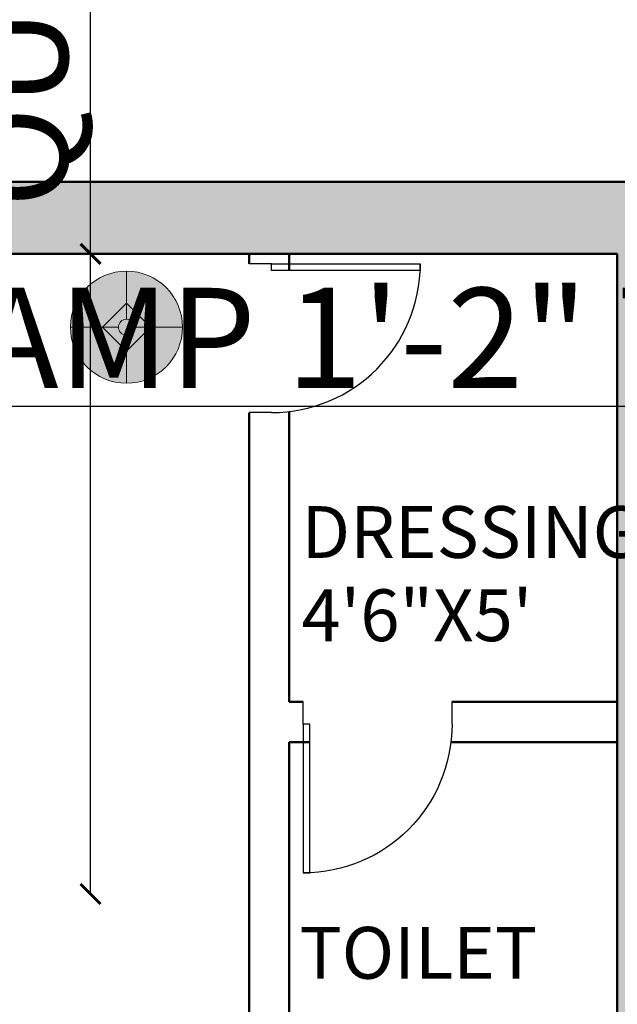
# Model space of a CAD drawing. Units: inches. Extents: x 2419 to 2878, y 1068 to 1713.
# Tile 18 of 20: x 2697 to 2772, y 1475 to 1598. Entities that reach past the tile are written whole.
import ezdxf

# ---------------------------------------------------------------- set-up
doc = ezdxf.new("R2010")
doc.units = ezdxf.units.IN
for name, color, linetype, lineweight in [('A-ANNO-DIMS', 2, 'Continuous', 18), ('A-AREA-IDEN', 7, 'Continuous', 18), ('A-DOOR', 4, 'Continuous', 25), ('A-FLOR-PRKG-PATT', 1, 'Continuous', 13), ('A-FURN', 8, 'Continuous', 18), ('A-FURN-PATT', 254, 'Continuous', 13), ('A-WALL', 7, 'Continuous', 50)]:
    doc.layers.add(name, color=color, linetype=linetype, lineweight=lineweight)
doc.layers.add('A-FLOR-FIXT-PATT', color=254, linetype='Continuous', lineweight=13, true_color=0xd7ebd2)
doc.layers.add('A-WALL-PATT', color=18, linetype='Continuous', lineweight=13, true_color=0x000000)
doc.styles.get("Standard").update_dxf_attribs({"font": 'arial.ttf'})
doc.dimstyles.new('ISO-25', dxfattribs={"dimtxt": 12.5, "dimasz": 2.5, "dimexe": 1.25, "dimexo": 0.625, "dimtad": 1, "dimdec": 0, "dimlunit": 4, "dimtxsty": 'Standard', "dimblk": 'ARCHTICK', "dimcen": 2.5, "dimse1": 1, "dimse2": 1, "dimclrd": 4, "dimadec": 0, "dimazin": 0, "dimtfac": 1, "dimtdec": 0, "dimtmove": 0, "dimatfit": 3, "dimfxl": 1, "dimarcsym": 0})

# ---------------------------------------------------------------- blocks, each defined once
blk = doc.blocks.new('*U3')
for p, q in [((0, 0), (0, -6)), ((40, 0), (40, -6))]:
    blk.add_line(p, q)
blk.add_lwpolyline([(0, 0), (0, 40), (1.75, 40), (1.75, 0)], close=True)
blk.add_arc((0, 0), 40, 0, 90)
blk = doc.blocks.new('Lamp - Table')
for p, q in [((0, 7), (0, 1)), ((0, 3), (-3, 0)), ((3, 0), (0, 3)), ((-1, 0), (-7, 0)), ((-3, 0), (0, -3)), ((0, -3), (3, 0)), ((1, 0), (7, 0)), ((0, -1), (0, -7))]:
    blk.add_line(p, q)
for radius in [7, 1]:
    blk.add_circle((0, 0), radius)
blk = doc.blocks.new('_ArchTick')
at = {"color": 0, "linetype": 'ByBlock', "const_width": 0.15}
blk.add_lwpolyline([(-0.5, -0.5), (0.5, 0.5)], dxfattribs=at)
blk = doc.blocks.new('*D16')
at = {"layer": 'A-ANNO-DIMS', "color": 0, "lineweight": -2, "transparency": 16777216}
blk.add_line((2471.51, 1623.24), (2780.51, 1623.24), dxfattribs=at)
at = {"layer": 'Defpoints', "color": 0, "transparency": 16777216}
for p in [(2780.51, 1623.24), (2471.51, 1577.81), (2780.51, 1577.81)]:
    blk.add_point(p, dxfattribs=at)
at = {"layer": 'A-ANNO-DIMS', "color": 0, "lineweight": -2, "transparency": 16777216, "xscale": 2.5, "yscale": 2.5, "zscale": 2.5, "rotation": 180}
blk.add_blockref('_ArchTick', (2471.51, 1623.24), dxfattribs=at)
at = {"layer": 'A-ANNO-DIMS', "color": 0, "lineweight": -2, "transparency": 16777216, "xscale": 2.5, "yscale": 2.5, "zscale": 2.5}
blk.add_blockref('_ArchTick', (2780.51, 1623.24), dxfattribs=at)
at = {"layer": 'A-ANNO-DIMS', "color": 0, "transparency": 16777216, "insert": (2626.01, 1630.25), "char_height": 12.5, "attachment_point": 5}
blk.add_mtext('25\'-9"', dxfattribs=at)
blk = doc.blocks.new('*D24')
at = {"layer": 'A-ANNO-DIMS', "color": 4, "lineweight": -2, "transparency": 16777216}
for p, q in [((2605.13, 1549.79), (2619.13, 1549.79)), ((2619.13, 1549.79), (2811.96, 1549.79))]:
    blk.add_line(p, q, dxfattribs=at)
at = {"layer": 'Defpoints', "color": 0, "transparency": 16777216}
for p in [(2605.13, 1551.89), (2619.13, 1551.89), (2619.13, 1549.79)]:
    blk.add_point(p, dxfattribs=at)
at = {"layer": 'A-ANNO-DIMS', "color": 4, "lineweight": -2, "transparency": 16777216, "xscale": 2.5, "yscale": 2.5, "zscale": 2.5, "rotation": 180}
blk.add_blockref('_ArchTick', (2605.13, 1549.79), dxfattribs=at)
at = {"layer": 'A-ANNO-DIMS', "color": 4, "lineweight": -2, "transparency": 16777216, "xscale": 2.5, "yscale": 2.5, "zscale": 2.5}
blk.add_blockref('_ArchTick', (2619.13, 1549.79), dxfattribs=at)
at = {"layer": 'A-ANNO-DIMS', "color": 0, "transparency": 16777216, "insert": (2716.8, 1556.69), "char_height": 12.5, "attachment_point": 5}
blk.add_mtext('TABLE LAMP 1\'-2" TYP.', dxfattribs=at)
blk = doc.blocks.new('*D30')
at = {"layer": 'A-ANNO-DIMS', "color": 4, "lineweight": -2, "transparency": 16777216}
for p, q in [((2705.68, 1568.81), (2705.68, 1713.47)), ((2705.68, 1488.81), (2705.68, 1568.81))]:
    blk.add_line(p, q, dxfattribs=at)
at = {"layer": 'Defpoints', "color": 0, "transparency": 16777216}
for p in [(2693.68, 1568.81), (2705.68, 1568.81), (2693.68, 1488.81)]:
    blk.add_point(p, dxfattribs=at)
at = {"layer": 'A-ANNO-DIMS', "color": 4, "lineweight": -2, "transparency": 16777216, "xscale": 2.5, "yscale": 2.5, "zscale": 2.5}
for p, rotation in [((2705.68, 1568.81), 90), ((2705.68, 1488.81), 270)]:
    blk.add_blockref('_ArchTick', p, dxfattribs=dict(at, rotation=rotation))
at = {"layer": 'A-ANNO-DIMS', "color": 0, "transparency": 16777216, "insert": (2698.21, 1642.39), "char_height": 12.5, "attachment_point": 5, "rotation": 90}
blk.add_mtext('QUEEN BED 6\'-8"', dxfattribs=at)
blk = doc.blocks.new('*D36')
at = {"layer": 'A-ANNO-DIMS', "color": 4, "lineweight": -2, "transparency": 16777216}
blk.add_line((2656.74, 1605.01), (2736.32, 1605.01), dxfattribs=at)
at = {"layer": 'Defpoints', "color": 0, "transparency": 16777216}
for p in [(2736.32, 1605.01), (2656.74, 1205.81), (2736.32, 1205.81)]:
    blk.add_point(p, dxfattribs=at)
at = {"layer": 'A-ANNO-DIMS', "color": 4, "lineweight": -2, "transparency": 16777216, "xscale": 2.5, "yscale": 2.5, "zscale": 2.5, "rotation": 180}
blk.add_blockref('_ArchTick', (2656.74, 1605.01), dxfattribs=at)
at = {"layer": 'A-ANNO-DIMS', "color": 4, "lineweight": -2, "transparency": 16777216, "xscale": 2.5, "yscale": 2.5, "zscale": 2.5}
blk.add_blockref('_ArchTick', (2736.32, 1605.01), dxfattribs=at)
at = {"layer": 'A-ANNO-DIMS', "color": 0, "transparency": 16777216, "insert": (2696.53, 1612.1), "char_height": 12.5, "attachment_point": 5}
blk.add_mtext('6\'-7 1/2"', dxfattribs=at)
blk = doc.blocks.new('*D37')
at = {"layer": 'A-ANNO-DIMS', "color": 4, "lineweight": -2, "transparency": 16777216}
for p, q in [((2736.32, 1605.01), (2771.51, 1605.01)), ((2771.51, 1605.01), (2818.42, 1605.01))]:
    blk.add_line(p, q, dxfattribs=at)
at = {"layer": 'Defpoints', "color": 0, "transparency": 16777216}
for p in [(2771.51, 1605.01), (2736.32, 1205.81), (2771.51, 1205.81)]:
    blk.add_point(p, dxfattribs=at)
at = {"layer": 'A-ANNO-DIMS', "color": 4, "lineweight": -2, "transparency": 16777216, "xscale": 2.5, "yscale": 2.5, "zscale": 2.5, "rotation": 180}
blk.add_blockref('_ArchTick', (2736.32, 1605.01), dxfattribs=at)
at = {"layer": 'A-ANNO-DIMS', "color": 4, "lineweight": -2, "transparency": 16777216, "xscale": 2.5, "yscale": 2.5, "zscale": 2.5}
blk.add_blockref('_ArchTick', (2771.51, 1605.01), dxfattribs=at)
at = {"layer": 'A-ANNO-DIMS', "color": 0, "transparency": 16777216, "insert": (2796.22, 1611.91), "char_height": 12.5, "attachment_point": 5}
blk.add_mtext('2\'-11"', dxfattribs=at)
blk = doc.blocks.new('*D39')
at = {"layer": 'A-ANNO-DIMS', "color": 4, "lineweight": -2, "transparency": 16777216}
for p, q in [((2662.74, 1605.01), (2668.59, 1605.01)), ((2668.59, 1605.01), (2705.56, 1605.01))]:
    blk.add_line(p, q, dxfattribs=at)
at = {"layer": 'Defpoints', "color": 0, "transparency": 16777216}
for p in [(2668.59, 1605.01), (2662.74, 1165.6), (2668.59, 1165.6)]:
    blk.add_point(p, dxfattribs=at)
at = {"layer": 'A-ANNO-DIMS', "color": 4, "lineweight": -2, "transparency": 16777216, "xscale": 2.5, "yscale": 2.5, "zscale": 2.5, "rotation": 180}
blk.add_blockref('_ArchTick', (2662.74, 1605.01), dxfattribs=at)
at = {"layer": 'A-ANNO-DIMS', "color": 4, "lineweight": -2, "transparency": 16777216, "xscale": 2.5, "yscale": 2.5, "zscale": 2.5}
blk.add_blockref('_ArchTick', (2668.59, 1605.01), dxfattribs=at)
at = {"layer": 'A-ANNO-DIMS', "color": 0, "transparency": 16777216, "insert": (2688.32, 1612.02), "char_height": 12.5, "attachment_point": 5}
blk.add_mtext('0\'-6"', dxfattribs=at)
blk = doc.blocks.new('*D48')
at = {"layer": 'A-ANNO-DIMS', "color": 4, "lineweight": -2, "transparency": 16777216}
for p, q in [((2444.31, 1567.55), (2444.31, 1548.96)), ((2444.31, 1548.96), (2444.31, 1484.03))]:
    blk.add_line(p, q, dxfattribs=at)
at = {"layer": 'Defpoints', "color": 0, "transparency": 16777216}
for p in [(2725.51, 1567.55), (2444.31, 1548.96), (2725.51, 1548.96)]:
    blk.add_point(p, dxfattribs=at)
at = {"layer": 'A-ANNO-DIMS', "color": 4, "lineweight": -2, "transparency": 16777216, "xscale": 2.5, "yscale": 2.5, "zscale": 2.5}
for p, rotation in [((2444.31, 1567.55), 90), ((2444.31, 1548.96), 270)]:
    blk.add_blockref('_ArchTick', p, dxfattribs=dict(at, rotation=rotation))
at = {"layer": 'A-ANNO-DIMS', "color": 0, "transparency": 16777216, "insert": (2437.23, 1515.25), "char_height": 12.5, "attachment_point": 5, "rotation": 90}
blk.add_mtext('1\'-6 1/2"', dxfattribs=at)
blk = doc.blocks.new('*D49')
at = {"layer": 'A-ANNO-DIMS', "color": 4, "lineweight": -2, "transparency": 16777216}
for p, q in [((2732.27, 1605.01), (2750.85, 1605.01)), ((2750.85, 1605.01), (2815.78, 1605.01))]:
    blk.add_line(p, q, dxfattribs=at)
at = {"layer": 'Defpoints', "color": 0, "transparency": 16777216}
for p in [(2750.85, 1605.01), (2732.27, 1512.81), (2750.85, 1512.81)]:
    blk.add_point(p, dxfattribs=at)
at = {"layer": 'A-ANNO-DIMS', "color": 4, "lineweight": -2, "transparency": 16777216, "xscale": 2.5, "yscale": 2.5, "zscale": 2.5, "rotation": 180}
blk.add_blockref('_ArchTick', (2732.27, 1605.01), dxfattribs=at)
at = {"layer": 'A-ANNO-DIMS', "color": 4, "lineweight": -2, "transparency": 16777216, "xscale": 2.5, "yscale": 2.5, "zscale": 2.5}
blk.add_blockref('_ArchTick', (2750.85, 1605.01), dxfattribs=at)
at = {"layer": 'A-ANNO-DIMS', "color": 0, "transparency": 16777216, "insert": (2784.57, 1612.1), "char_height": 12.5, "attachment_point": 5}
blk.add_mtext('1\'-6 1/2"', dxfattribs=at)
blk = doc.blocks.new('*D50')
at = {"layer": 'A-ANNO-DIMS', "color": 4, "lineweight": -2, "transparency": 16777216}
for p, q in [((2444.31, 1458.39), (2444.31, 1494.19)), ((2444.31, 1437.39), (2444.31, 1458.39))]:
    blk.add_line(p, q, dxfattribs=at)
at = {"layer": 'Defpoints', "color": 0, "transparency": 16777216}
for p in [(2444.31, 1458.39), (2763.51, 1458.39), (2763.51, 1437.39)]:
    blk.add_point(p, dxfattribs=at)
at = {"layer": 'A-ANNO-DIMS', "color": 4, "lineweight": -2, "transparency": 16777216, "xscale": 2.5, "yscale": 2.5, "zscale": 2.5}
for p, rotation in [((2444.31, 1458.39), 90), ((2444.31, 1437.39), 270)]:
    blk.add_blockref('_ArchTick', p, dxfattribs=dict(at, rotation=rotation))
at = {"layer": 'A-ANNO-DIMS', "color": 0, "transparency": 16777216, "insert": (2437.31, 1477.54), "char_height": 12.5, "attachment_point": 5, "rotation": 90}
blk.add_mtext('1\'-9"', dxfattribs=at)
blk = doc.blocks.new('*D53')
at = {"layer": 'A-ANNO-DIMS', "color": 4, "lineweight": -2, "transparency": 16777216}
for p, q in [((2638.79, 1605.01), (2667.31, 1605.01)), ((2667.31, 1605.01), (2733.63, 1605.01))]:
    blk.add_line(p, q, dxfattribs=at)
at = {"layer": 'Defpoints', "color": 0, "transparency": 16777216}
for p in [(2667.31, 1605.01), (2638.79, 1217.38), (2667.31, 1217.38)]:
    blk.add_point(p, dxfattribs=at)
at = {"layer": 'A-ANNO-DIMS', "color": 4, "lineweight": -2, "transparency": 16777216, "xscale": 2.5, "yscale": 2.5, "zscale": 2.5, "rotation": 180}
blk.add_blockref('_ArchTick', (2638.79, 1605.01), dxfattribs=at)
at = {"layer": 'A-ANNO-DIMS', "color": 4, "lineweight": -2, "transparency": 16777216, "xscale": 2.5, "yscale": 2.5, "zscale": 2.5}
blk.add_blockref('_ArchTick', (2667.31, 1605.01), dxfattribs=at)
at = {"layer": 'A-ANNO-DIMS', "color": 0, "transparency": 16777216, "insert": (2701.72, 1612.1), "char_height": 12.5, "attachment_point": 5}
blk.add_mtext('2\'-4 1/2"', dxfattribs=at)

msp = doc.modelspace()

# ---------------------------------------------------------------- hatches: boundary and pattern name
at = {"layer": 'A-FLOR-FIXT-PATT'}
h = msp.add_hatch(color=256, dxfattribs=at)
h.dxf.hatch_style = 1
h.paths.add_polyline_path([(2771.51, 1458.39), (2763.51, 1458.39), (2763.51, 1437.39), (2771.51, 1437.39)])
h.paths.add_polyline_path([(2770.51, 1456.39, 0.5), (2769.51, 1457.39), (2765.51, 1457.39, 0.5), (2764.51, 1456.39), (2764.51, 1439.39, 0.5), (2765.51, 1438.39), (2769.51, 1438.39, 0.5), (2770.51, 1439.39)], flags=16)
h.paths.add_polyline_path([(2706.38, 1408.81), (2685.38, 1408.81), (2685.38, 1400.81), (2706.38, 1400.81)])
h.paths.add_polyline_path([(2704.38, 1401.81, 0.5), (2705.38, 1402.81), (2705.38, 1406.81, 0.5), (2704.38, 1407.81), (2687.38, 1407.81, 0.5), (2686.38, 1406.81), (2686.38, 1402.81, 0.5), (2687.38, 1401.81)], flags=16)
h.paths.add_polyline_path([(2574.48, 1207.45), (2633.94, 1207.45), (2633.94, 1217.37), (2574.48, 1217.37)], flags=9)
h.paths.add_polyline_path([(2574.45, 1217.83), (2610.47, 1217.83), (2610.47, 1227.88), (2574.45, 1227.88)], flags=9)
h.paths.add_polyline_path([(2672.43, 1304.02), (2718.62, 1304.02), (2718.62, 1313.94), (2672.43, 1313.94)], flags=9)
h.paths.add_polyline_path([(2672.4, 1314.4), (2750.13, 1314.4), (2750.13, 1324.45), (2672.4, 1324.45)], flags=9)
h.paths.add_polyline_path([(2500.43, 1374.44), (2544.8, 1374.44), (2544.8, 1384.36), (2500.43, 1384.36)], flags=9)
h.paths.add_polyline_path([(2500.41, 1384.82), (2566.08, 1384.82), (2566.08, 1394.87), (2500.41, 1394.87)], flags=9)
h.paths.add_polyline_path([(2738.93, 1376.75), (2778.27, 1376.75), (2778.27, 1386.67), (2738.93, 1386.67)], flags=9)
h.paths.add_polyline_path([(2659.12, 1357.8), (2703.49, 1357.8), (2703.49, 1367.72), (2659.12, 1367.72)], flags=9)
h.paths.add_polyline_path([(2659.1, 1368.18), (2694.11, 1368.18), (2694.11, 1378.23), (2659.1, 1378.23)], flags=9)
h.paths.add_polyline_path([(2730.12, 1466.07), (2769.46, 1466.07), (2769.46, 1475.99), (2730.12, 1475.99)], flags=9)
h.paths.add_polyline_path([(2730.1, 1476.45), (2765.12, 1476.45), (2765.12, 1486.5), (2730.1, 1486.5)], flags=9)
h.paths.add_polyline_path([(2730.38, 1518.65), (2761.48, 1518.65), (2761.48, 1528.57), (2730.38, 1528.57)], flags=9)
h.paths.add_polyline_path([(2730.36, 1529.03), (2780.96, 1529.03), (2780.96, 1539.07), (2730.36, 1539.07)], flags=9)
h.paths.add_polyline_path([(2629.32, 1455.19), (2688.78, 1455.19), (2688.78, 1465.11), (2629.32, 1465.11)], flags=9)
h.paths.add_polyline_path([(2629.3, 1465.57), (2681.9, 1465.57), (2681.9, 1475.62), (2629.3, 1475.62)], flags=9)
h.paths.add_polyline_path([(2513.23, 1456.48), (2562.63, 1456.48), (2562.63, 1466.4), (2513.23, 1466.4)], flags=9)
h.paths.add_polyline_path([(2513.21, 1466.86), (2556.26, 1466.86), (2556.26, 1476.91), (2513.21, 1476.91)], flags=9)
h.paths.add_polyline_path([(2488.87, 1521.54), (2519.97, 1521.54), (2519.97, 1531.46), (2488.87, 1531.46)], flags=9)
h.paths.add_polyline_path([(2536.55, 1543.51), (2580.92, 1543.51), (2580.92, 1553.43), (2536.55, 1553.43)], flags=9)
h.paths.add_polyline_path([(2536.56, 1553.92), (2573.53, 1553.92), (2573.53, 1563.8), (2536.56, 1563.8)], flags=9)
at = {"layer": 'A-FLOR-PRKG-PATT'}
h = msp.add_hatch(color=256, dxfattribs=at)
h.dxf.hatch_style = 1
edge = h.paths.add_edge_path()
edge.add_ellipse((2561.37, 1279.45), major_axis=(3.99, 0), ratio=0.842304, start_angle=0.6466, end_angle=90)
edge.add_line((2561.37, 1282.81), (2511.57, 1282.81))
edge.add_ellipse((2511.57, 1279.45), major_axis=(3.99, 0), ratio=0.842304, start_angle=90, end_angle=179.3534)
edge.add_ellipse((10560.89, 1188.62), major_axis=(-8054.03, 0), ratio=0.8423039, start_angle=-0.646554, end_angle=-0.628237)
edge.add_ellipse((2509.23, 1276.91), major_axis=(1.69, 0), ratio=0.842304, start_angle=179.3718, end_angle=248.4648)
edge.add_ellipse((10560.33, 1188.62), major_axis=(8052.29, 0), ratio=0.8423039, start_angle=179.353446, end_angle=179.381357, ccw=False)
edge.add_ellipse((2511.01, 1279.45), major_axis=(2.25, 0), ratio=0.842304, start_angle=90, end_angle=179.3534, ccw=False)
edge.add_line((2511.01, 1281.35), (2561.94, 1281.35))
edge.add_ellipse((2561.94, 1279.45), major_axis=(-2.25, 0), ratio=0.842304, start_angle=180.6466, end_angle=270, ccw=False)
edge.add_ellipse((-5487.38, 1188.62), major_axis=(8052.29, 0), ratio=0.8423039, start_angle=0.528271, end_angle=0.646554, ccw=False)
edge.add_ellipse((2563.71, 1276.91), major_axis=(-1.69, 0), ratio=0.842304, start_angle=111.5352, end_angle=180.6282)
edge.add_ellipse((-5487.95, 1188.62), major_axis=(-8054.03, 0), ratio=0.8423039, start_angle=180.628237, end_angle=180.646554)
edge = h.paths.add_edge_path()
edge.add_ellipse((2564.91, 1261.91), major_axis=(-1.12, 0), ratio=0.842304, start_angle=180, end_angle=270)
edge.add_line((2564.91, 1262.86), (2564.43, 1262.86))
edge.add_ellipse((-5487.38, 1188.62), major_axis=(8052.29, 0), ratio=0.8423039, start_angle=0.383867, end_angle=0.528271, ccw=False)
edge.add_line((2564.65, 1242.56), (2564.91, 1242.56))
edge.add_ellipse((2564.91, 1243.51), major_axis=(-1.12, 0), ratio=0.842304, start_angle=90, end_angle=180)
edge.add_line((2566.03, 1243.51), (2566.03, 1261.91))
edge = h.paths.add_edge_path()
edge.add_ellipse((2564.91, 1174.99), major_axis=(1.12, 0), ratio=0.842304, start_angle=0, end_angle=90)
edge.add_line((2564.91, 1175.94), (2564.89, 1175.94))
edge.add_ellipse((-5487.38, 1188.62), major_axis=(8052.29, 0), ratio=0.8423039, start_angle=-0.134987, end_angle=-0.090229, ccw=False)
edge.add_ellipse((2163.34, 1170.91), major_axis=(401.54, 0), ratio=0.842304, start_angle=-2.18, end_angle=-0.1356, ccw=False)
edge.add_line((2564.47, 1155.64), (2564.91, 1155.64))
edge.add_ellipse((2564.91, 1156.59), major_axis=(-1.12, 0), ratio=0.842304, start_angle=90, end_angle=180)
edge.add_line((2566.03, 1156.59), (2566.03, 1174.99))
h.paths.add_polyline_path([(2574.48, 1207.45), (2633.94, 1207.45), (2633.94, 1217.37), (2574.48, 1217.37)], flags=9)
h.paths.add_polyline_path([(2574.45, 1217.83), (2610.47, 1217.83), (2610.47, 1227.88), (2574.45, 1227.88)], flags=9)
h.paths.add_polyline_path([(2672.43, 1304.02), (2718.62, 1304.02), (2718.62, 1313.94), (2672.43, 1313.94)], flags=9)
h.paths.add_polyline_path([(2672.4, 1314.4), (2750.13, 1314.4), (2750.13, 1324.45), (2672.4, 1324.45)], flags=9)
h.paths.add_polyline_path([(2500.43, 1374.44), (2544.8, 1374.44), (2544.8, 1384.36), (2500.43, 1384.36)], flags=9)
h.paths.add_polyline_path([(2500.41, 1384.82), (2566.08, 1384.82), (2566.08, 1394.87), (2500.41, 1394.87)], flags=9)
h.paths.add_polyline_path([(2738.93, 1376.75), (2778.27, 1376.75), (2778.27, 1386.67), (2738.93, 1386.67)], flags=9)
h.paths.add_polyline_path([(2659.12, 1357.8), (2703.49, 1357.8), (2703.49, 1367.72), (2659.12, 1367.72)], flags=9)
h.paths.add_polyline_path([(2659.1, 1368.18), (2694.11, 1368.18), (2694.11, 1378.23), (2659.1, 1378.23)], flags=9)
h.paths.add_polyline_path([(2730.12, 1466.07), (2769.46, 1466.07), (2769.46, 1475.99), (2730.12, 1475.99)], flags=9)
h.paths.add_polyline_path([(2730.1, 1476.45), (2765.12, 1476.45), (2765.12, 1486.5), (2730.1, 1486.5)], flags=9)
h.paths.add_polyline_path([(2730.38, 1518.65), (2761.48, 1518.65), (2761.48, 1528.57), (2730.38, 1528.57)], flags=9)
h.paths.add_polyline_path([(2730.36, 1529.03), (2780.96, 1529.03), (2780.96, 1539.07), (2730.36, 1539.07)], flags=9)
h.paths.add_polyline_path([(2629.32, 1455.19), (2688.78, 1455.19), (2688.78, 1465.11), (2629.32, 1465.11)], flags=9)
h.paths.add_polyline_path([(2629.3, 1465.57), (2681.9, 1465.57), (2681.9, 1475.62), (2629.3, 1475.62)], flags=9)
h.paths.add_polyline_path([(2513.23, 1456.48), (2562.63, 1456.48), (2562.63, 1466.4), (2513.23, 1466.4)], flags=9)
h.paths.add_polyline_path([(2513.21, 1466.86), (2556.26, 1466.86), (2556.26, 1476.91), (2513.21, 1476.91)], flags=9)
h.paths.add_polyline_path([(2488.87, 1521.54), (2519.97, 1521.54), (2519.97, 1531.46), (2488.87, 1531.46)], flags=9)
h.paths.add_polyline_path([(2536.55, 1543.51), (2580.92, 1543.51), (2580.92, 1553.43), (2536.55, 1553.43)], flags=9)
h.paths.add_polyline_path([(2536.56, 1553.92), (2573.53, 1553.92), (2573.53, 1563.8), (2536.56, 1563.8)], flags=9)
at = {"layer": 'A-FURN-PATT'}
h = msp.add_hatch(color=256, dxfattribs=at)
h.dxf.hatch_style = 1
h.paths.add_polyline_path([(2619.13, 1558.89), (2615.13, 1558.89), (2612.13, 1555.89), (2612.13, 1551.89, 0.414214)])
h.paths.add_polyline_path([(2612.13, 1565.89), (2612.13, 1561.89), (2615.13, 1558.89), (2619.13, 1558.89, 0.414214)])
h.paths.add_polyline_path([(2612.13, 1561.89), (2612.13, 1565.89, 0.414214), (2605.13, 1558.89), (2609.13, 1558.89)])
h.paths.add_polyline_path([(2612.13, 1555.89), (2609.13, 1558.89), (2605.13, 1558.89, 0.414214), (2612.13, 1551.89)])
h.paths.add_polyline_path([(2710.17, 1562.64), (2710.17, 1566.64, 0.414214), (2703.17, 1559.64), (2707.17, 1559.64)])
h.paths.add_polyline_path([(2710.17, 1556.64), (2707.17, 1559.64), (2703.17, 1559.64, 0.414214), (2710.17, 1552.64)])
h.paths.add_polyline_path([(2717.17, 1559.64), (2713.17, 1559.64), (2710.17, 1556.64), (2710.17, 1552.64, 0.414214)])
h.paths.add_polyline_path([(2710.17, 1566.64), (2710.17, 1562.64), (2713.17, 1559.64), (2717.17, 1559.64, 0.414214)])
h = msp.add_hatch(color=256, dxfattribs=at)
h.dxf.hatch_style = 1
h.paths.add_polyline_path([(2710.17, 1562.64), (2707.17, 1559.64), (2709.17, 1559.64, -0.414214), (2710.17, 1560.64)])
h.paths.add_polyline_path([(2711.17, 1559.64, 1), (2709.17, 1559.64, 1)])
h.paths.add_polyline_path([(2710.17, 1562.64), (2710.17, 1560.64, -0.414214), (2711.17, 1559.64), (2713.17, 1559.64)])
h.paths.add_polyline_path([(2713.17, 1559.64), (2711.17, 1559.64, -0.414214), (2710.17, 1558.64), (2710.17, 1556.64)])
h.paths.add_polyline_path([(2710.17, 1558.64, -0.414214), (2709.17, 1559.64), (2707.17, 1559.64), (2710.17, 1556.64)])
h.paths.add_polyline_path([(2613.13, 1558.89, 1), (2611.13, 1558.89, 1)])
h.paths.add_polyline_path([(2612.13, 1561.89), (2612.13, 1559.89, -0.414214), (2613.13, 1558.89), (2615.13, 1558.89)])
h.paths.add_polyline_path([(2612.13, 1559.89), (2612.13, 1561.89), (2609.13, 1558.89), (2611.13, 1558.89, -0.414214)])
h.paths.add_polyline_path([(2612.13, 1557.89, -0.414214), (2611.13, 1558.89), (2609.13, 1558.89), (2612.13, 1555.89)])
h.paths.add_polyline_path([(2574.48, 1207.45), (2633.94, 1207.45), (2633.94, 1217.37), (2574.48, 1217.37)], flags=9)
h.paths.add_polyline_path([(2574.45, 1217.83), (2610.47, 1217.83), (2610.47, 1227.88), (2574.45, 1227.88)], flags=9)
h.paths.add_polyline_path([(2672.43, 1304.02), (2718.62, 1304.02), (2718.62, 1313.94), (2672.43, 1313.94)], flags=9)
h.paths.add_polyline_path([(2672.4, 1314.4), (2750.13, 1314.4), (2750.13, 1324.45), (2672.4, 1324.45)], flags=9)
h.paths.add_polyline_path([(2500.43, 1374.44), (2544.8, 1374.44), (2544.8, 1384.36), (2500.43, 1384.36)], flags=9)
h.paths.add_polyline_path([(2500.41, 1384.82), (2566.08, 1384.82), (2566.08, 1394.87), (2500.41, 1394.87)], flags=9)
h.paths.add_polyline_path([(2738.93, 1376.75), (2778.27, 1376.75), (2778.27, 1386.67), (2738.93, 1386.67)], flags=9)
h.paths.add_polyline_path([(2659.12, 1357.8), (2703.49, 1357.8), (2703.49, 1367.72), (2659.12, 1367.72)], flags=9)
h.paths.add_polyline_path([(2659.1, 1368.18), (2694.11, 1368.18), (2694.11, 1378.23), (2659.1, 1378.23)], flags=9)
h.paths.add_polyline_path([(2730.12, 1466.07), (2769.46, 1466.07), (2769.46, 1475.99), (2730.12, 1475.99)], flags=9)
h.paths.add_polyline_path([(2730.1, 1476.45), (2765.12, 1476.45), (2765.12, 1486.5), (2730.1, 1486.5)], flags=9)
h.paths.add_polyline_path([(2730.38, 1518.65), (2761.48, 1518.65), (2761.48, 1528.57), (2730.38, 1528.57)], flags=9)
h.paths.add_polyline_path([(2730.36, 1529.03), (2780.96, 1529.03), (2780.96, 1539.07), (2730.36, 1539.07)], flags=9)
h.paths.add_polyline_path([(2629.32, 1455.19), (2688.78, 1455.19), (2688.78, 1465.11), (2629.32, 1465.11)], flags=9)
h.paths.add_polyline_path([(2629.3, 1465.57), (2681.9, 1465.57), (2681.9, 1475.62), (2629.3, 1475.62)], flags=9)
h.paths.add_polyline_path([(2513.23, 1456.48), (2562.63, 1456.48), (2562.63, 1466.4), (2513.23, 1466.4)], flags=9)
h.paths.add_polyline_path([(2513.21, 1466.86), (2556.26, 1466.86), (2556.26, 1476.91), (2513.21, 1476.91)], flags=9)
h.paths.add_polyline_path([(2488.87, 1521.54), (2519.97, 1521.54), (2519.97, 1531.46), (2488.87, 1531.46)], flags=9)
h.paths.add_polyline_path([(2536.55, 1543.51), (2580.92, 1543.51), (2580.92, 1553.43), (2536.55, 1553.43)], flags=9)
h.paths.add_polyline_path([(2536.56, 1553.92), (2573.53, 1553.92), (2573.53, 1563.8), (2536.56, 1563.8)], flags=9)
at = {"layer": 'A-WALL-PATT'}
h = msp.add_hatch(color=256, dxfattribs=at)
h.dxf.hatch_style = 1
h.paths.add_polyline_path([(2780.51, 1577.81), (2471.51, 1577.81), (2471.51, 1121.81), (2780.51, 1121.81)])
h.paths.add_polyline_path([(2480.51, 1568.81), (2771.51, 1568.81), (2771.51, 1130.81), (2480.51, 1130.81)], flags=16)
h.paths.add_polyline_path([(2528.51, 1568.81), (2528.51, 1512.81), (2594.51, 1512.81), (2594.51, 1414.81), (2596.57, 1414.81), (2596.57, 1441.61), (2597.82, 1441.61), (2597.82, 1441.58, -0.384016), (2625.03, 1414.81), (2725.51, 1414.81), (2725.51, 1567.55), (2728.3, 1567.55), (2746.89, 1567.55), (2746.89, 1566.73), (2746.87, 1566.73, -0.367216), (2730.51, 1549.09), (2730.51, 1512.81), (2750.85, 1512.81), (2750.85, 1510.03, -0.401453), (2733.08, 1491.46), (2733.08, 1491.44), (2732.27, 1491.44), (2732.27, 1507.81), (2730.51, 1507.81), (2730.51, 1408.81), (2736.51, 1408.81), (2736.51, 1349.81), (2632.51, 1349.81), (2632.51, 1408.81), (2528.51, 1408.81), (2528.51, 1414.81), (2503.97, 1414.81), (2503.97, 1494.85), (2558.38, 1494.85), (2558.38, 1507.81), (2529.96, 1507.81, -0.414214), (2530.82, 1506.96), (2530.82, 1497.26, -0.414214), (2529.96, 1496.4), (2514.56, 1496.4, -0.414214), (2513.7, 1497.26), (2513.7, 1506.96, -0.414214), (2514.56, 1507.81), (2528.51, 1507.81), (2528.51, 1512.81), (2480.51, 1512.81)], flags=0)
h.paths.add_polyline_path([(2516.26, 1507.81), (2528.26, 1507.81), (2528.26, 1505.81), (2523.42, 1505.81), (2524.07, 1504.67), (2529.39, 1504.67, -0.414214), (2529.96, 1504.1), (2529.96, 1497.83, -0.414214), (2529.39, 1497.26), (2515.13, 1497.26, -0.414214), (2514.56, 1497.83), (2514.56, 1504.1, -0.414214), (2515.13, 1504.67), (2520.69, 1504.67), (2521.34, 1505.81), (2516.26, 1505.81)], flags=0)
h.paths.add_polyline_path([(2522.02, 1505.53), (2522.82, 1507.32, -0.65506), (2522.25, 1506.06), (2522.19, 1505.93), (2522.43, 1505.53)], flags=0)
h.paths.add_polyline_path([(2522.83, 1500.97, -1), (2521.69, 1500.97, -1)], flags=0)
h.paths.add_polyline_path([(2522.55, 1500.97, -1), (2521.98, 1500.97, -1)], flags=0)
h.paths.add_polyline_path([(2482.01, 1470.63), (2499.89, 1470.63), (2499.89, 1448.27), (2482.01, 1448.27), (2482.01, 1452.74), (2481.26, 1452.74), (2481.26, 1449.76), (2480.51, 1449.76), (2480.51, 1469.14), (2481.26, 1469.14), (2481.26, 1466.16), (2482.01, 1466.16)], flags=0)
h.paths.add_polyline_path([(2488.71, 1466.16, -1), (2484.24, 1466.16, -1)], flags=0)
h.paths.add_polyline_path([(2496.17, 1466.16, -1), (2490.2, 1466.16, -1)], flags=0)
h.paths.add_polyline_path([(2487.97, 1466.16, -1), (2484.99, 1466.16, -1)], flags=0)
h.paths.add_polyline_path([(2495.42, 1466.16, -1), (2490.95, 1466.16, -1)], flags=0)
h.paths.add_polyline_path([(2487.22, 1466.16, -1), (2485.73, 1466.16, -1)], flags=0)
h.paths.add_polyline_path([(2494.68, 1466.16, -1), (2491.69, 1466.16, -1)], flags=0)
h.paths.add_polyline_path([(2499.11, 1468, -1), (2497.98, 1468, -1)], flags=0)
h.paths.add_polyline_path([(2493.93, 1466.16, -1), (2492.44, 1466.16, -1)], flags=0)
h.paths.add_polyline_path([(2499.37, 1463.71, -1), (2498.17, 1463.71, -1)], flags=0)
h.paths.add_polyline_path([(2484.24, 1461.69), (2496.17, 1461.69), (2496.17, 1457.22), (2484.24, 1457.22)], flags=0)
h.paths.add_polyline_path([(2484.99, 1460.94), (2495.42, 1460.94), (2495.42, 1457.96), (2484.99, 1457.96)], flags=0)
h.paths.add_polyline_path([(2586.88, 1510.03), (2587.69, 1510.03), (2587.69, 1491.44), (2586.88, 1491.44)], flags=0)
h.paths.add_polyline_path([(2499.26, 1459.41, -1), (2498.2, 1459.41, -1)], flags=0)
h.paths.add_polyline_path([(2489.46, 1452.74, -1), (2483.5, 1452.74, -1)], flags=0)
h.paths.add_polyline_path([(2557.3, 1408.81), (2557.3, 1413.09, -0.401453), (2584.57, 1441.58), (2584.57, 1441.61), (2585.82, 1441.61), (2585.82, 1413.09), (2585.82, 1408.81)], flags=0)
h.paths.add_polyline_path([(2488.71, 1452.74, -1), (2484.24, 1452.74, -1)], flags=0)
h.paths.add_polyline_path([(2495.42, 1452.74, -1), (2490.95, 1452.74, -1)], flags=0)
h.paths.add_polyline_path([(2487.97, 1452.74, -1), (2484.99, 1452.74, -1)], flags=0)
h.paths.add_polyline_path([(2494.68, 1452.74, -1), (2491.69, 1452.74, -1)], flags=0)
h.paths.add_polyline_path([(2487.22, 1452.74, -1), (2485.73, 1452.74, -1)], flags=0)
h.paths.add_polyline_path([(2499.18, 1454.44, -1), (2497.9, 1454.44, -1)], flags=0)
h.paths.add_polyline_path([(2493.93, 1452.74, -1), (2492.44, 1452.74, -1)], flags=0)
h.paths.add_polyline_path([(2499.3, 1450.64, -1), (2497.79, 1450.64, -1)], flags=0)
h.paths.add_polyline_path([(2619.13, 1558.89, -1), (2605.13, 1558.89, -1)], flags=0)
h.paths.add_polyline_path([(2609.13, 1558.89), (2612.13, 1561.89), (2615.13, 1558.89), (2612.13, 1555.89)], flags=0)
h.paths.add_polyline_path([(2611.13, 1558.89, -1), (2613.13, 1558.89, -1)], flags=0)
h.paths.add_polyline_path([(2633.68, 1568.81), (2693.68, 1568.81), (2693.68, 1488.81), (2633.68, 1488.81)], flags=0)
h.paths.add_polyline_path([(2641.68, 1554.41), (2641.68, 1567.61), (2662.48, 1567.61), (2662.48, 1554.41), (2664.88, 1554.41), (2664.88, 1567.61), (2685.68, 1567.61), (2685.68, 1552.41), (2680.48, 1552.41), (2693.68, 1539.21), (2678.48, 1539.21), (2678.48, 1554.41)], flags=0)
h.paths.add_polyline_path([(2637.51, 1408.81), (2731.51, 1408.81), (2731.51, 1354.81), (2637.51, 1354.81), (2637.51, 1357.98), (2635.3, 1357.98), (2635.3, 1358.79), (2637.51, 1358.79)], flags=0)
h.paths.add_polyline_path([(2717.17, 1559.64, -1), (2703.17, 1559.64, -1)], flags=0)
h.paths.add_polyline_path([(2707.17, 1559.64), (2710.17, 1562.64), (2713.17, 1559.64), (2710.17, 1556.64)], flags=0)
h.paths.add_polyline_path([(2709.17, 1559.64, -1), (2711.17, 1559.64, -1)], flags=0)
h.paths.add_polyline_path([(2685.38, 1408.81), (2706.38, 1408.81), (2706.38, 1400.81), (2699.88, 1400.81), (2701.88, 1394.81, -0.501323), (2696.92, 1375.95, -0.132891), (2694.83, 1375.95, -0.501317), (2689.88, 1394.81), (2691.88, 1400.81), (2688.88, 1400.81), (2688.88, 1399.31), (2685.88, 1399.31), (2685.88, 1400.31), (2687.88, 1400.31), (2687.88, 1400.81), (2685.38, 1400.81)], flags=0)
h.paths.add_polyline_path([(2687.38, 1407.81), (2704.38, 1407.81, -0.5), (2705.38, 1406.81), (2705.38, 1402.81, -0.5), (2704.38, 1401.81), (2687.38, 1401.81, -0.5), (2686.38, 1402.81), (2686.38, 1406.81, -0.5)], flags=0)
h.paths.add_polyline_path([(2639.51, 1205.81), (2634.51, 1205.81), (2634.51, 1293.81), (2637.51, 1293.81), (2639.51, 1293.81)], flags=0)
h.paths.add_polyline_path([(2691.88, 1394.81), (2699.88, 1394.81, -0.48008), (2697.52, 1377.29, -0.215004), (2694.23, 1377.29, -0.48008)], flags=0)
h.paths.add_polyline_path([(2757.51, 1453.89), (2763.51, 1451.89), (2763.51, 1454.89), (2762.01, 1454.89), (2762.01, 1457.89), (2763.01, 1457.89), (2763.01, 1455.89), (2763.51, 1455.89), (2763.51, 1458.39), (2771.51, 1458.39), (2771.51, 1437.39), (2763.51, 1437.39), (2763.51, 1443.89), (2757.51, 1441.89, -0.501323), (2738.65, 1446.85, -0.132891), (2738.65, 1448.94, -0.501317)], flags=0)
h.paths.add_polyline_path([(2739.99, 1449.54, -0.48008), (2757.51, 1451.89), (2757.51, 1443.89, -0.48008), (2739.99, 1446.25, -0.215004)], flags=0)
h.paths.add_polyline_path([(2765.51, 1457.39), (2769.51, 1457.39, -0.5), (2770.51, 1456.39), (2770.51, 1439.39, -0.5), (2769.51, 1438.39), (2765.51, 1438.39, -0.5), (2764.51, 1439.39), (2764.51, 1456.39, -0.5)], flags=0)
h = msp.add_hatch(color=256, dxfattribs=at)
h.dxf.hatch_style = 1
h.paths.add_polyline_path([(2771.51, 1354.81), (2736.51, 1354.81), (2736.51, 1408.81), (2771.51, 1408.81), (2771.51, 1414.81), (2625.03, 1414.81, -0.015108), (2625.09, 1413.09), (2625.09, 1408.81), (2632.51, 1408.81), (2632.51, 1376.56), (2635.3, 1376.56, -0.029838), (2637.51, 1376.43), (2637.51, 1408.81), (2731.51, 1408.81), (2731.51, 1354.81), (2637.51, 1354.81), (2637.51, 1357.98), (2635.3, 1357.98), (2632.51, 1357.98), (2632.51, 1349.81), (2771.51, 1349.81)])
h.paths.add_polyline_path([(2639.51, 1298.81), (2637.51, 1298.81), (2480.51, 1298.81), (2480.51, 1293.81), (2637.51, 1293.81), (2639.51, 1293.81)])
h.paths.add_polyline_path([(2639.51, 1293.81), (2637.51, 1293.81), (2634.51, 1293.81), (2634.51, 1244.65), (2638.79, 1244.65, -0.006332), (2639.51, 1244.64)])
h.paths.add_polyline_path([(2639.51, 1205.81), (2771.51, 1205.81), (2771.51, 1210.81), (2639.51, 1210.81), (2639.51, 1216.13), (2638.79, 1216.13), (2634.51, 1216.13), (2634.51, 1130.81), (2639.51, 1130.81)])
h.paths.add_polyline_path([(2596.57, 1413.09), (2596.57, 1414.81), (2585.82, 1414.81), (2585.82, 1413.09), (2585.82, 1408.81), (2596.57, 1408.81)])
h.paths.add_polyline_path([(2557.3, 1413.09, -0.015108), (2557.35, 1414.81), (2480.51, 1414.81), (2480.51, 1408.81), (2557.3, 1408.81)])
h.paths.add_polyline_path([(2574.48, 1207.45), (2633.94, 1207.45), (2633.94, 1217.37), (2574.48, 1217.37)], flags=9)
h.paths.add_polyline_path([(2574.45, 1217.83), (2610.47, 1217.83), (2610.47, 1227.88), (2574.45, 1227.88)], flags=9)
h.paths.add_polyline_path([(2672.43, 1304.02), (2718.62, 1304.02), (2718.62, 1313.94), (2672.43, 1313.94)], flags=9)
h.paths.add_polyline_path([(2672.4, 1314.4), (2750.13, 1314.4), (2750.13, 1324.45), (2672.4, 1324.45)], flags=9)
h.paths.add_polyline_path([(2500.43, 1374.44), (2544.8, 1374.44), (2544.8, 1384.36), (2500.43, 1384.36)], flags=9)
h.paths.add_polyline_path([(2500.41, 1384.82), (2566.08, 1384.82), (2566.08, 1394.87), (2500.41, 1394.87)], flags=9)
h.paths.add_polyline_path([(2738.93, 1376.75), (2778.27, 1376.75), (2778.27, 1386.67), (2738.93, 1386.67)], flags=9)
h.paths.add_polyline_path([(2659.12, 1357.8), (2703.49, 1357.8), (2703.49, 1367.72), (2659.12, 1367.72)], flags=25)
h.paths.add_polyline_path([(2659.1, 1368.18), (2694.11, 1368.18), (2694.11, 1378.23), (2659.1, 1378.23)], flags=25)
h.paths.add_polyline_path([(2730.12, 1466.07), (2769.46, 1466.07), (2769.46, 1475.99), (2730.12, 1475.99)], flags=9)
h.paths.add_polyline_path([(2730.1, 1476.45), (2765.12, 1476.45), (2765.12, 1486.5), (2730.1, 1486.5)], flags=9)
h.paths.add_polyline_path([(2730.38, 1518.65), (2761.48, 1518.65), (2761.48, 1528.57), (2730.38, 1528.57)], flags=9)
h.paths.add_polyline_path([(2730.36, 1529.03), (2780.96, 1529.03), (2780.96, 1539.07), (2730.36, 1539.07)], flags=9)
h.paths.add_polyline_path([(2629.32, 1455.19), (2688.78, 1455.19), (2688.78, 1465.11), (2629.32, 1465.11)], flags=9)
h.paths.add_polyline_path([(2629.3, 1465.57), (2681.9, 1465.57), (2681.9, 1475.62), (2629.3, 1475.62)], flags=9)
h.paths.add_polyline_path([(2513.23, 1456.48), (2562.63, 1456.48), (2562.63, 1466.4), (2513.23, 1466.4)], flags=9)
h.paths.add_polyline_path([(2513.21, 1466.86), (2556.26, 1466.86), (2556.26, 1476.91), (2513.21, 1476.91)], flags=9)
h.paths.add_polyline_path([(2488.87, 1521.54), (2519.97, 1521.54), (2519.97, 1531.46), (2488.87, 1531.46)], flags=9)
h.paths.add_polyline_path([(2536.55, 1543.51), (2580.92, 1543.51), (2580.92, 1553.43), (2536.55, 1553.43)], flags=9)
h.paths.add_polyline_path([(2536.56, 1553.92), (2573.53, 1553.92), (2573.53, 1563.8), (2536.56, 1563.8)], flags=9)

# ---------------------------------------------------------------- linework, layer by layer
at = {"layer": 'A-WALL'}
for p, q in [((2480.51, 1568.81), (2771.51, 1568.81)), ((2725.51, 1567.55), (2725.51, 1568.81)), ((2730.51, 1566.73), (2730.51, 1568.81)), ((2771.51, 1568.81), (2771.51, 1130.81)), ((2725.51, 1414.81), (2725.51, 1548.96)), ((2730.51, 1512.81), (2730.51, 1549.09)), ((2730.51, 1512.81), (2732.27, 1512.81)), ((2750.85, 1512.81), (2771.51, 1512.81)), ((2730.51, 1414.81), (2730.51, 1507.81)), ((2730.51, 1507.81), (2733.08, 1507.81)), ((2750.72, 1507.81), (2771.51, 1507.81))]:
    msp.add_line(p, q, dxfattribs=at)
msp.add_lwpolyline([(2471.51, 1577.81), (2780.51, 1577.81), (2780.51, 1121.81), (2471.51, 1121.81)], close=True, dxfattribs=at)

# ---------------------------------------------------------------- block references
at = {"layer": 'A-DOOR', "yscale": 0.4646269055216028, "zscale": 0.4646269055216028}
for p, xscale, rotation in [((2728.3, 1567.55), 0.4646269055216028, 270), ((2732.27, 1510.03), -0.4646269055216028, 180)]:
    msp.add_blockref('*U3', p, dxfattribs=dict(at, xscale=xscale, rotation=rotation))
at = {"layer": 'A-FURN'}
msp.add_blockref('Lamp - Table', (2710.17, 1559.64), dxfattribs=at)

# ---------------------------------------------------------------- texts
at = {"layer": 'A-AREA-IDEN'}
for s, p in [('DRESSING', (2732.04, 1530.81)), ('4\'6"X5\'', (2732.04, 1520.41)), ('TOILET', (2731.78, 1478.23))]:
    msp.add_text(s, height=6.475, dxfattribs=at).set_placement(p)

# ---------------------------------------------------------------- dimensions: what is measured, and where the dimension line sits
at = {"layer": 'A-ANNO-DIMS'}
dim = msp.add_linear_dim(base=(2705.68, 1568.81), p1=(2693.68, 1488.81), p2=(2693.68, 1568.81), angle=90, text='QUEEN BED <>', dimstyle='ISO-25', override={"dimdec": 1, "dimlfac": 1, "dimrnd": 0, "dimzin": 1, "dimdsep": 46, "dimlunit": 4, "dimfrac": 2}, dxfattribs=at)
dim.commit()
dim.dimension.update_dxf_attribs({"geometry": '*D30', "text_midpoint": (2698.21, 1642.39)})
for base, p1, p2, override, picture, middle in [((2780.51, 1623.24), (2471.51, 1577.81), (2780.51, 1577.81), {"dimclrd": 0, "dimclre": 0, "dimclrt": 0}, '*D16', (2626.01, 1630.25)), ((2667.31, 1605.01), (2638.79, 1217.38), (2667.31, 1217.38), {"dimdec": 1, "dimlfac": 1, "dimrnd": 0, "dimzin": 1, "dimdsep": 46, "dimlunit": 4, "dimfrac": 2}, '*D53', (2701.72, 1612.1)), ((2736.32, 1605.01), (2656.74, 1205.81), (2736.32, 1205.81), {"dimdec": 1, "dimlfac": 1, "dimrnd": 0, "dimzin": 1, "dimdsep": 46, "dimlunit": 4, "dimfrac": 2}, '*D36', (2696.53, 1612.1)), ((2750.85, 1605.01), (2732.27, 1512.81), (2750.85, 1512.81), {"dimdec": 1, "dimlfac": 1, "dimrnd": 0, "dimzin": 1, "dimdsep": 46, "dimlunit": 4, "dimfrac": 2}, '*D49', (2784.57, 1612.1)), ((2668.5856, 1605.013), (2662.7408, 1165.6026), (2668.5856, 1165.6026), {"dimdec": 1, "dimlfac": 1, "dimrnd": 0, "dimzin": 1, "dimdsep": 46, "dimlunit": 4, "dimfrac": 2}, '*D39', (2688.3247, 1612.0201)), ((2771.51, 1605.01), (2736.32, 1205.81), (2771.51, 1205.81), {"dimdec": 1, "dimlfac": 1, "dimrnd": 0, "dimzin": 1, "dimdsep": 46, "dimlunit": 4, "dimfrac": 2}, '*D37', (2796.22, 1611.91))]:
    dim = msp.add_linear_dim(base=base, p1=p1, p2=p2, dimstyle='ISO-25', override=override, dxfattribs=at)
    dim.commit()
    dim.dimension.update_dxf_attribs({"geometry": picture, "text_midpoint": middle})
dim = msp.add_linear_dim(base=(2619.13, 1549.79), p1=(2605.13, 1551.89), p2=(2619.13, 1551.89), text='TABLE LAMP <> TYP.', dimstyle='ISO-25', override={"dimdec": 1, "dimlfac": 1, "dimrnd": 0, "dimzin": 1, "dimdsep": 46, "dimlunit": 4, "dimfrac": 2}, dxfattribs=at)
dim.commit()
dim.dimension.update_dxf_attribs({"geometry": '*D24', "text_midpoint": (2716.8, 1556.69)})
for base, p1, p2, picture, middle in [((2444.31, 1548.96), (2725.51, 1567.55), (2725.51, 1548.96), '*D48', (2437.23, 1515.25)), ((2444.31, 1458.39), (2763.51, 1437.39), (2763.51, 1458.39), '*D50', (2437.31, 1477.54))]:
    dim = msp.add_linear_dim(base=base, p1=p1, p2=p2, angle=90, dimstyle='ISO-25', override={"dimdec": 1, "dimlfac": 1, "dimrnd": 0, "dimzin": 1, "dimdsep": 46, "dimlunit": 4, "dimfrac": 2}, dxfattribs=at)
    dim.commit()
    dim.dimension.update_dxf_attribs({"geometry": picture, "text_midpoint": middle})

doc.saveas('drawing.dxf')
